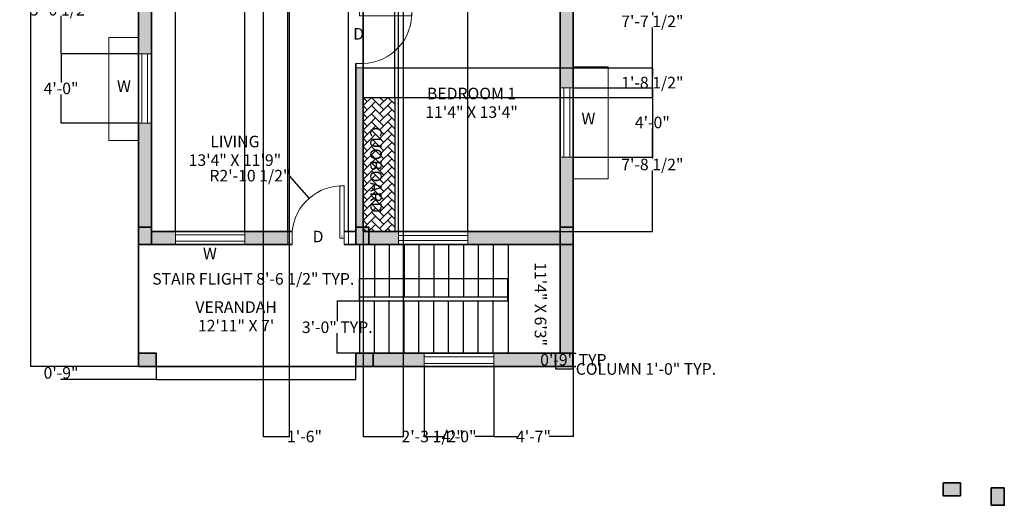
# Model space of a CAD drawing. Units: inches. Extents: x 374 to 1054, y -870 to -188.
# Tile 1 of 3: x 374 to 1054, y -870 to -535. Entities that reach past the tile are written whole.
import ezdxf
from ezdxf.enums import TextEntityAlignment as Align

# ---------------------------------------------------------------- set-up
doc = ezdxf.new("R2010")
doc.units = ezdxf.units.IN
doc.header["$MEASUREMENT"] = 0
for name, color, linetype, lineweight, true_color in [('A-ANNO-DIMS', 244, 'Continuous', 18, 0x991b1e), ('A-AREA-IDEN', 116, 'Continuous', 18, 0x136734), ('A-WALL-PATT', 116, 'Continuous', 13, 0x136734)]:
    doc.layers.add(name, color=color, linetype=linetype, lineweight=lineweight, true_color=true_color)
for name, color, linetype, lineweight in [('A-ANNO-SYMB', 6, 'Continuous', 18), ('A-ANNO-TEXT', 7, 'Continuous', 18), ('A-COLS', 1, 'Continuous', 35), ('A-DOOR', 4, 'Continuous', 18), ('A-FLOR-CASE', 8, 'Continuous', 25), ('A-FLOR-CASE-PATT', 8, 'Continuous', 13), ('A-FLOR-STRS', 7, 'Continuous', 25), ('A-GLAZ', 4, 'Continuous', 18), ('A-GLAZ-PROJ', 4, 'Continuous', 13), ('A-WALL', 7, 'Continuous', 35)]:
    doc.layers.add(name, color=color, linetype=linetype, lineweight=lineweight)
doc.styles.get("Standard").update_dxf_attribs({"font": 'arial.ttf'})
doc.dimstyles.get("Standard").update_dxf_attribs({"dimtxt": 8, "dimasz": 0.18, "dimexe": 0.18, "dimexo": 0.0625, "dimgap": 0.09, "dimtad": 0, "dimtih": 1, "dimtoh": 1, "dimzin": 0, "dimdsep": 46, "dimlunit": 3, "dimtxsty": 'Standard', "dimcen": 0.09, "dimadec": 0, "dimazin": 0, "dimtfac": 1, "dimtofl": 0, "dimtmove": 0, "dimatfit": 3, "dimfxl": 1, "dimtolj": 1, "dimtzin": 0, "dimarcsym": 0})

# ---------------------------------------------------------------- blocks, each defined once
blk = doc.blocks.new('*D2')
at = {"layer": 'A-ANNO-DIMS', "color": 0, "lineweight": -2, "transparency": 16777216}
for p, q in [((455.84, -257.94), (381.2, -257.94)), ((381.38, -258.12), (381.38, -511.76)), ((381.38, -773.76), (381.38, -520.12)), ((455.84, -773.94), (381.2, -773.94))]:
    blk.add_line(p, q, dxfattribs=at)
at = {"layer": 'A-ANNO-DIMS', "color": 0, "transparency": 16777216}
for points in [[(381.35, -258.12), (381.41, -258.12), (381.38, -257.94)], [(381.35, -773.76), (381.41, -773.76), (381.38, -773.94)]]:
    blk.add_solid(points, dxfattribs=at)
at = {"layer": 'Defpoints', "color": 0, "transparency": 16777216}
for p in [(381.38, -257.94), (455.9, -257.94), (455.9, -773.94)]:
    blk.add_point(p, dxfattribs=at)
at = {"layer": 'A-ANNO-DIMS', "color": 0, "transparency": 16777216, "insert": (381.38, -515.94), "char_height": 8, "attachment_point": 5}
blk.add_mtext("\\A1;43'", dxfattribs=at)
blk = doc.blocks.new('COL-12X9')
h = blk.add_hatch(color=256)
h.dxf.hatch_style = 1
h.paths.add_polyline_path([(6, 4.5), (-6, 4.5), (-6, -4.5), (6, -4.5)])
blk.add_lwpolyline([(-6, 4.5), (6, 4.5), (6, -4.5), (-6, -4.5)], close=True)
blk = doc.blocks.new('DOOR-SWING-36')
blk.add_lwpolyline([(0, 0), (-3, 0), (-3, 36), (0, 36)], close=True)
blk.add_arc((-1.5, 1.52), 34.51, 87.5091, 178.37068)
blk = doc.blocks.new('STAIR-FLIGHT-36')
for p, q in [((10.25, 36), (10.25, 0)), ((20.5, 36), (20.5, 0)), ((30.75, 36), (30.75, 0)), ((41, 36), (41, 0)), ((51.25, 36), (51.25, 0)), ((61.5, 36), (61.5, 0)), ((71.75, 36), (71.75, 0)), ((82, 36), (82, 0)), ((92.25, 36), (92.25, 0)), ((0, 0), (102.5, 0))]:
    blk.add_line(p, q)
blk = doc.blocks.new('*D6')
at = {"layer": 'A-ANNO-DIMS', "color": 0, "lineweight": -2, "transparency": 16777216}
for p, q in [((743.74, -774), (743.74, -775.92)), ((755.74, -774), (755.74, -775.92)), ((743.92, -775.74), (755.56, -775.74)), ((755.74, -775.74), (755.92, -775.74))]:
    blk.add_line(p, q, dxfattribs=at)
at = {"layer": 'A-ANNO-DIMS', "color": 0, "transparency": 16777216}
for points in [[(743.92, -775.71), (743.92, -775.77), (743.74, -775.74)], [(755.56, -775.71), (755.56, -775.77), (755.74, -775.74)]]:
    blk.add_solid(points, dxfattribs=at)
at = {"layer": 'Defpoints', "color": 0, "transparency": 16777216}
for p in [(743.74, -773.94), (755.74, -773.94), (755.74, -775.74)]:
    blk.add_point(p, dxfattribs=at)
at = {"layer": 'A-ANNO-DIMS', "color": 0, "transparency": 16777216, "insert": (806.11, -775.74), "char_height": 8, "attachment_point": 5}
blk.add_mtext('\\A1;COLUMN 1\'-0" TYP.', dxfattribs=at)
blk = doc.blocks.new('*D7')
at = {"layer": 'A-ANNO-DIMS', "color": 0, "lineweight": -2, "transparency": 16777216}
for p, q in [((755.8, -764.94), (757.72, -764.94)), ((757.54, -765.12), (757.54, -765.26)), ((755.8, -773.94), (757.72, -773.94)), ((757.54, -773.76), (757.54, -773.61))]:
    blk.add_line(p, q, dxfattribs=at)
at = {"layer": 'A-ANNO-DIMS', "color": 0, "transparency": 16777216}
for points in [[(757.51, -765.12), (757.57, -765.12), (757.54, -764.94)], [(757.51, -773.76), (757.57, -773.76), (757.54, -773.94)]]:
    blk.add_solid(points, dxfattribs=at)
at = {"layer": 'Defpoints', "color": 0, "transparency": 16777216}
for p in [(755.74, -764.94), (757.54, -764.94), (755.74, -773.94)]:
    blk.add_point(p, dxfattribs=at)
at = {"layer": 'A-ANNO-DIMS', "color": 0, "transparency": 16777216, "insert": (757.54, -769.44), "char_height": 8, "attachment_point": 5}
blk.add_mtext('\\A1;0\'-9" TYP.', dxfattribs=at)
blk = doc.blocks.new('*D10')
at = {"layer": 'A-ANNO-DIMS', "color": 0, "lineweight": -2, "transparency": 16777216}
for p, q in [((608.4, -713.56), (608.22, -713.56)), ((608.4, -728.88), (608.4, -713.38)), ((710.72, -713.56), (608.58, -713.56)), ((710.9, -728.88), (710.9, -713.38))]:
    blk.add_line(p, q, dxfattribs=at)
at = {"layer": 'A-ANNO-DIMS', "color": 0, "transparency": 16777216}
for points in [[(608.58, -713.53), (608.58, -713.59), (608.4, -713.56)], [(710.72, -713.53), (710.72, -713.59), (710.9, -713.56)]]:
    blk.add_solid(points, dxfattribs=at)
at = {"layer": 'Defpoints', "color": 0, "transparency": 16777216}
for p in [(608.4, -713.56), (608.4, -728.94), (710.9, -728.94)]:
    blk.add_point(p, dxfattribs=at)
at = {"layer": 'A-ANNO-DIMS', "color": 0, "transparency": 16777216, "insert": (535.02, -713.56), "char_height": 8, "attachment_point": 5}
blk.add_mtext('\\A1;STAIR FLIGHT 8\'-6 1/2" TYP.', dxfattribs=at)
blk = doc.blocks.new('*D11')
at = {"layer": 'A-ANNO-DIMS', "color": 0, "lineweight": -2, "transparency": 16777216}
for p, q in [((608.34, -728.94), (592.85, -728.94)), ((593.03, -729.12), (593.03, -742.76)), ((593.03, -764.76), (593.03, -751.12)), ((608.34, -764.94), (592.85, -764.94))]:
    blk.add_line(p, q, dxfattribs=at)
at = {"layer": 'A-ANNO-DIMS', "color": 0, "transparency": 16777216}
for points in [[(593, -729.12), (593.06, -729.12), (593.03, -728.94)], [(593, -764.76), (593.06, -764.76), (593.03, -764.94)]]:
    blk.add_solid(points, dxfattribs=at)
at = {"layer": 'Defpoints', "color": 0, "transparency": 16777216}
for p in [(608.4, -728.94), (593.03, -764.94), (608.4, -764.94)]:
    blk.add_point(p, dxfattribs=at)
at = {"layer": 'A-ANNO-DIMS', "color": 0, "transparency": 16777216, "insert": (593.03, -746.94), "char_height": 8, "attachment_point": 5}
blk.add_mtext('\\A1;3\'-0" TYP.', dxfattribs=at)
blk = doc.blocks.new('*D22')
at = {"layer": 'A-ANNO-DIMS', "color": 0, "lineweight": -2, "transparency": 16777216}
for p, q in [((455.84, -497.43), (402.18, -497.43)), ((402.36, -497.61), (402.36, -523.56)), ((402.36, -557.96), (402.36, -532.01)), ((455.84, -558.14), (402.18, -558.14))]:
    blk.add_line(p, q, dxfattribs=at)
at = {"layer": 'A-ANNO-DIMS', "color": 0, "transparency": 16777216}
for points in [[(402.33, -497.61), (402.39, -497.61), (402.36, -497.43)], [(402.33, -557.96), (402.39, -557.96), (402.36, -558.14)]]:
    blk.add_solid(points, dxfattribs=at)
at = {"layer": 'Defpoints', "color": 0, "transparency": 16777216}
for p in [(455.9, -497.43), (402.36, -558.14), (455.9, -558.14)]:
    blk.add_point(p, dxfattribs=at)
at = {"layer": 'A-ANNO-DIMS', "color": 0, "transparency": 16777216, "insert": (402.36, -527.79), "char_height": 8, "attachment_point": 5}
blk.add_mtext('\\A1;5\'-0 1/2"', dxfattribs=at)
blk = doc.blocks.new('*D23')
at = {"layer": 'A-ANNO-DIMS', "color": 0, "lineweight": -2, "transparency": 16777216}
for p, q in [((455.84, -558.14), (402.18, -558.14)), ((402.36, -558.32), (402.36, -577.97)), ((402.36, -605.96), (402.36, -586.31)), ((455.84, -606.14), (402.18, -606.14))]:
    blk.add_line(p, q, dxfattribs=at)
at = {"layer": 'A-ANNO-DIMS', "color": 0, "transparency": 16777216}
for points in [[(402.33, -558.32), (402.39, -558.32), (402.36, -558.14)], [(402.33, -605.96), (402.39, -605.96), (402.36, -606.14)]]:
    blk.add_solid(points, dxfattribs=at)
at = {"layer": 'Defpoints', "color": 0, "transparency": 16777216}
for p in [(455.9, -558.14), (402.36, -606.14), (455.9, -606.14)]:
    blk.add_point(p, dxfattribs=at)
at = {"layer": 'A-ANNO-DIMS', "color": 0, "transparency": 16777216, "insert": (402.36, -582.14), "char_height": 8, "attachment_point": 5}
blk.add_mtext('\\A1;4\'-0"', dxfattribs=at)
blk = doc.blocks.new('*D30')
at = {"layer": 'A-ANNO-DIMS', "color": 0, "lineweight": -2, "transparency": 16777216}
for p, q in [((755.97, -489.99), (810.73, -489.99)), ((810.55, -490.17), (810.55, -531.58)), ((810.55, -581.43), (810.55, -540.03)), ((755.97, -581.61), (810.73, -581.61))]:
    blk.add_line(p, q, dxfattribs=at)
at = {"layer": 'A-ANNO-DIMS', "color": 0, "transparency": 16777216}
for points in [[(810.52, -490.17), (810.58, -490.17), (810.55, -489.99)], [(810.52, -581.43), (810.58, -581.43), (810.55, -581.61)]]:
    blk.add_solid(points, dxfattribs=at)
at = {"layer": 'Defpoints', "color": 0, "transparency": 16777216}
for p in [(755.9, -489.99), (755.9, -581.61), (810.55, -581.61)]:
    blk.add_point(p, dxfattribs=at)
at = {"layer": 'A-ANNO-DIMS', "color": 0, "transparency": 16777216, "insert": (810.55, -535.8), "char_height": 8, "attachment_point": 5}
blk.add_mtext('\\A1;7\'-7 1/2"', dxfattribs=at)
blk = doc.blocks.new('*D31')
at = {"layer": 'A-ANNO-DIMS', "color": 0, "lineweight": -2, "transparency": 16777216}
for p, q in [((755.97, -581.61), (810.73, -581.61)), ((810.55, -581.79), (810.55, -601.44)), ((810.55, -629.43), (810.55, -609.79)), ((755.97, -629.61), (810.73, -629.61))]:
    blk.add_line(p, q, dxfattribs=at)
at = {"layer": 'A-ANNO-DIMS', "color": 0, "transparency": 16777216}
for points in [[(810.52, -581.79), (810.58, -581.79), (810.55, -581.61)], [(810.52, -629.43), (810.58, -629.43), (810.55, -629.61)]]:
    blk.add_solid(points, dxfattribs=at)
at = {"layer": 'Defpoints', "color": 0, "transparency": 16777216}
for p in [(755.9, -581.61), (755.9, -629.61), (810.55, -629.61)]:
    blk.add_point(p, dxfattribs=at)
at = {"layer": 'A-ANNO-DIMS', "color": 0, "transparency": 16777216, "insert": (810.55, -605.61), "char_height": 8, "attachment_point": 5}
blk.add_mtext('\\A1;4\'-0"', dxfattribs=at)
blk = doc.blocks.new('*D32')
at = {"layer": 'A-ANNO-DIMS', "color": 0, "lineweight": -2, "transparency": 16777216}
for p, q in [((701.11, -774), (701.11, -822.55)), ((755.9, -774), (755.9, -822.55)), ((701.29, -822.37), (717.62, -822.37)), ((755.72, -822.37), (739.39, -822.37))]:
    blk.add_line(p, q, dxfattribs=at)
at = {"layer": 'A-ANNO-DIMS', "color": 0, "transparency": 16777216}
for points in [[(701.29, -822.34), (701.29, -822.4), (701.11, -822.37)], [(755.72, -822.34), (755.72, -822.4), (755.9, -822.37)]]:
    blk.add_solid(points, dxfattribs=at)
at = {"layer": 'Defpoints', "color": 0, "transparency": 16777216}
for p in [(701.11, -773.94), (755.9, -773.94), (701.11, -822.37)]:
    blk.add_point(p, dxfattribs=at)
at = {"layer": 'A-ANNO-DIMS', "color": 0, "transparency": 16777216, "insert": (728.5, -822.37), "char_height": 8, "attachment_point": 5}
blk.add_mtext('\\A1;4\'-7"', dxfattribs=at)
blk = doc.blocks.new('*D33')
at = {"layer": 'A-ANNO-DIMS', "color": 0, "lineweight": -2, "transparency": 16777216}
for p, q in [((653.11, -774), (653.11, -822.55)), ((701.11, -774), (701.11, -822.55)), ((653.29, -822.37), (666.22, -822.37)), ((700.93, -822.37), (687.99, -822.37))]:
    blk.add_line(p, q, dxfattribs=at)
at = {"layer": 'A-ANNO-DIMS', "color": 0, "transparency": 16777216}
for points in [[(653.29, -822.34), (653.29, -822.4), (653.11, -822.37)], [(700.93, -822.34), (700.93, -822.4), (701.11, -822.37)]]:
    blk.add_solid(points, dxfattribs=at)
at = {"layer": 'Defpoints', "color": 0, "transparency": 16777216}
for p in [(653.11, -773.94), (701.11, -773.94), (653.11, -822.37)]:
    blk.add_point(p, dxfattribs=at)
at = {"layer": 'A-ANNO-DIMS', "color": 0, "transparency": 16777216, "insert": (677.11, -822.37), "char_height": 8, "attachment_point": 5}
blk.add_mtext('\\A1;4\'-0"', dxfattribs=at)
blk = doc.blocks.new('*D34')
at = {"layer": 'A-ANNO-DIMS', "color": 0, "lineweight": -2, "transparency": 16777216}
for p, q in [((467.84, -773.94), (402.18, -773.94)), ((402.36, -774.12), (402.36, -774.26)), ((467.84, -782.94), (402.18, -782.94)), ((402.36, -782.76), (402.36, -782.61))]:
    blk.add_line(p, q, dxfattribs=at)
at = {"layer": 'A-ANNO-DIMS', "color": 0, "transparency": 16777216}
for points in [[(402.33, -774.12), (402.39, -774.12), (402.36, -773.94)], [(402.33, -782.76), (402.39, -782.76), (402.36, -782.94)]]:
    blk.add_solid(points, dxfattribs=at)
at = {"layer": 'Defpoints', "color": 0, "transparency": 16777216}
for p in [(402.36, -773.94), (467.9, -773.94), (467.9, -782.94)]:
    blk.add_point(p, dxfattribs=at)
at = {"layer": 'A-ANNO-DIMS', "color": 0, "transparency": 16777216, "insert": (402.36, -778.44), "char_height": 8, "attachment_point": 5}
blk.add_mtext('\\A1;0\'-9"', dxfattribs=at)
blk = doc.blocks.new('*D35')
at = {"layer": 'A-ANNO-DIMS', "color": 0, "lineweight": -2, "transparency": 16777216}
for p, q in [((610.9, -361.5), (610.9, -822.55)), ((638.56, -361.5), (638.56, -822.55)), ((611.08, -822.37), (638.38, -822.37)), ((638.56, -822.37), (638.74, -822.37))]:
    blk.add_line(p, q, dxfattribs=at)
at = {"layer": 'A-ANNO-DIMS', "color": 0, "transparency": 16777216}
for points in [[(611.08, -822.34), (611.08, -822.4), (610.9, -822.37)], [(638.38, -822.34), (638.38, -822.4), (638.56, -822.37)]]:
    blk.add_solid(points, dxfattribs=at)
at = {"layer": 'Defpoints', "color": 0, "transparency": 16777216}
for p in [(610.9, -361.44), (638.56, -361.44), (638.56, -822.37)]:
    blk.add_point(p, dxfattribs=at)
at = {"layer": 'A-ANNO-DIMS', "color": 0, "transparency": 16777216, "insert": (658.85, -822.37), "char_height": 8, "attachment_point": 5}
blk.add_mtext('\\A1;2\'-3 1/2"', dxfattribs=at)
blk = doc.blocks.new('*D37')
at = {"layer": 'A-ANNO-DIMS', "color": 0, "lineweight": -2, "transparency": 16777216}
for p, q in [((610.9, -588.25), (610.9, -207.66)), ((611.08, -207.84), (632.5, -207.84)), ((632.68, -588.25), (632.68, -207.66)), ((632.68, -207.84), (632.86, -207.84))]:
    blk.add_line(p, q, dxfattribs=at)
at = {"layer": 'A-ANNO-DIMS', "color": 0, "transparency": 16777216}
for points in [[(611.08, -207.81), (611.08, -207.87), (610.9, -207.84)], [(632.5, -207.81), (632.5, -207.87), (632.68, -207.84)]]:
    blk.add_solid(points, dxfattribs=at)
at = {"layer": 'Defpoints', "color": 0, "transparency": 16777216}
for p in [(632.68, -207.84), (610.9, -588.31), (632.68, -588.31)]:
    blk.add_point(p, dxfattribs=at)
at = {"layer": 'A-ANNO-DIMS', "color": 0, "transparency": 16777216, "insert": (646.31, -207.84), "char_height": 8, "attachment_point": 5}
blk.add_mtext('\\A1;1\'-10"', dxfattribs=at)
blk = doc.blocks.new('*D38')
at = {"layer": 'A-ANNO-DIMS', "color": 0, "lineweight": -2, "transparency": 16777216}
for p, q in [((632.74, -588.31), (810.73, -588.31)), ((810.55, -588.49), (810.55, -630.4)), ((810.55, -680.76), (810.55, -638.85)), ((632.74, -680.94), (810.73, -680.94))]:
    blk.add_line(p, q, dxfattribs=at)
at = {"layer": 'A-ANNO-DIMS', "color": 0, "transparency": 16777216}
for points in [[(810.52, -588.49), (810.58, -588.49), (810.55, -588.31)], [(810.52, -680.76), (810.58, -680.76), (810.55, -680.94)]]:
    blk.add_solid(points, dxfattribs=at)
at = {"layer": 'Defpoints', "color": 0, "transparency": 16777216}
for p in [(632.68, -588.31), (632.68, -680.94), (810.55, -680.94)]:
    blk.add_point(p, dxfattribs=at)
at = {"layer": 'A-ANNO-DIMS', "color": 0, "transparency": 16777216, "insert": (810.55, -634.63), "char_height": 8, "attachment_point": 5}
blk.add_mtext('\\A1;7\'-8 1/2"', dxfattribs=at)
blk = doc.blocks.new('*D39')
at = {"layer": 'A-ANNO-DIMS', "color": 0, "lineweight": -2, "transparency": 16777216}
for p, q in [((464.9, -680.88), (464.9, -207.66)), ((465.08, -207.84), (481.13, -207.84)), ((481.31, -680.88), (481.31, -207.66)), ((481.31, -207.84), (481.49, -207.84))]:
    blk.add_line(p, q, dxfattribs=at)
at = {"layer": 'A-ANNO-DIMS', "color": 0, "transparency": 16777216}
for points in [[(465.08, -207.81), (465.08, -207.87), (464.9, -207.84)], [(481.13, -207.81), (481.13, -207.87), (481.31, -207.84)]]:
    blk.add_solid(points, dxfattribs=at)
at = {"layer": 'Defpoints', "color": 0, "transparency": 16777216}
for p in [(481.31, -207.84), (464.9, -680.94), (481.31, -680.94)]:
    blk.add_point(p, dxfattribs=at)
at = {"layer": 'A-ANNO-DIMS', "color": 0, "transparency": 16777216, "insert": (501.16, -207.84), "char_height": 8, "attachment_point": 5}
blk.add_mtext('\\A1;1\'-4 1/2"', dxfattribs=at)
blk = doc.blocks.new('*D40')
at = {"layer": 'A-ANNO-DIMS', "color": 0, "lineweight": -2, "transparency": 16777216}
for p, q in [((481.31, -680.88), (481.31, -207.66)), ((481.49, -207.84), (494.43, -207.84)), ((529.13, -207.84), (516.2, -207.84)), ((529.31, -680.88), (529.31, -207.66))]:
    blk.add_line(p, q, dxfattribs=at)
at = {"layer": 'A-ANNO-DIMS', "color": 0, "transparency": 16777216}
for points in [[(481.49, -207.81), (481.49, -207.87), (481.31, -207.84)], [(529.13, -207.81), (529.13, -207.87), (529.31, -207.84)]]:
    blk.add_solid(points, dxfattribs=at)
at = {"layer": 'Defpoints', "color": 0, "transparency": 16777216}
for p in [(529.31, -207.84), (481.31, -680.94), (529.31, -680.94)]:
    blk.add_point(p, dxfattribs=at)
at = {"layer": 'A-ANNO-DIMS', "color": 0, "transparency": 16777216, "insert": (505.31, -207.84), "char_height": 8, "attachment_point": 5}
blk.add_mtext('\\A1;4\'-0"', dxfattribs=at)
blk = doc.blocks.new('*D41')
at = {"layer": 'A-ANNO-DIMS', "color": 0, "lineweight": -2, "transparency": 16777216}
for p, q in [((529.31, -680.88), (529.31, -207.66)), ((529.49, -207.84), (558.72, -207.84)), ((558.9, -680.88), (558.9, -207.66)), ((558.9, -207.84), (559.08, -207.84))]:
    blk.add_line(p, q, dxfattribs=at)
at = {"layer": 'A-ANNO-DIMS', "color": 0, "transparency": 16777216}
for points in [[(529.49, -207.81), (529.49, -207.87), (529.31, -207.84)], [(558.72, -207.81), (558.72, -207.87), (558.9, -207.84)]]:
    blk.add_solid(points, dxfattribs=at)
at = {"layer": 'Defpoints', "color": 0, "transparency": 16777216}
for p in [(558.9, -207.84), (529.31, -680.94), (558.9, -680.94)]:
    blk.add_point(p, dxfattribs=at)
at = {"layer": 'A-ANNO-DIMS', "color": 0, "transparency": 16777216, "insert": (579.2, -207.84), "char_height": 8, "attachment_point": 5}
blk.add_mtext('\\A1;2\'-5 1/2"', dxfattribs=at)
blk = doc.blocks.new('*D42')
at = {"layer": 'A-ANNO-DIMS', "color": 0, "lineweight": -2, "transparency": 16777216}
for p, q in [((558.9, -680.88), (558.9, -207.66)), ((559.08, -207.84), (569.18, -207.84)), ((600.72, -207.84), (590.63, -207.84)), ((600.9, -680.88), (600.9, -207.66))]:
    blk.add_line(p, q, dxfattribs=at)
at = {"layer": 'A-ANNO-DIMS', "color": 0, "transparency": 16777216}
for points in [[(559.08, -207.81), (559.08, -207.87), (558.9, -207.84)], [(600.72, -207.81), (600.72, -207.87), (600.9, -207.84)]]:
    blk.add_solid(points, dxfattribs=at)
at = {"layer": 'Defpoints', "color": 0, "transparency": 16777216}
for p in [(600.9, -207.84), (558.9, -680.94), (600.9, -680.94)]:
    blk.add_point(p, dxfattribs=at)
at = {"layer": 'A-ANNO-DIMS', "color": 0, "transparency": 16777216, "insert": (579.9, -207.84), "char_height": 8, "attachment_point": 5}
blk.add_mtext('\\A1;3\'-6"', dxfattribs=at)
blk = doc.blocks.new('*D43')
at = {"layer": 'A-ANNO-DIMS', "color": 0, "lineweight": -2, "transparency": 16777216}
for p, q in [((635.25, -680.88), (635.25, -207.66)), ((635.43, -207.84), (648.36, -207.84)), ((683.07, -207.84), (670.13, -207.84)), ((683.25, -680.88), (683.25, -207.66))]:
    blk.add_line(p, q, dxfattribs=at)
at = {"layer": 'A-ANNO-DIMS', "color": 0, "transparency": 16777216}
for points in [[(635.43, -207.81), (635.43, -207.87), (635.25, -207.84)], [(683.07, -207.81), (683.07, -207.87), (683.25, -207.84)]]:
    blk.add_solid(points, dxfattribs=at)
at = {"layer": 'Defpoints', "color": 0, "transparency": 16777216}
for p in [(683.25, -207.84), (635.25, -680.94), (683.25, -680.94)]:
    blk.add_point(p, dxfattribs=at)
at = {"layer": 'A-ANNO-DIMS', "color": 0, "transparency": 16777216, "insert": (659.25, -207.84), "char_height": 8, "attachment_point": 5}
blk.add_mtext('\\A1;4\'-0"', dxfattribs=at)
blk = doc.blocks.new('*D44')
at = {"layer": 'A-ANNO-DIMS', "color": 0, "lineweight": -2, "transparency": 16777216}
for p, q in [((683.25, -680.88), (683.25, -207.66)), ((683.43, -207.84), (695.03, -207.84)), ((746.72, -207.84), (735.12, -207.84)), ((746.9, -680.88), (746.9, -207.66))]:
    blk.add_line(p, q, dxfattribs=at)
at = {"layer": 'A-ANNO-DIMS', "color": 0, "transparency": 16777216}
for points in [[(683.43, -207.81), (683.43, -207.87), (683.25, -207.84)], [(746.72, -207.81), (746.72, -207.87), (746.9, -207.84)]]:
    blk.add_solid(points, dxfattribs=at)
at = {"layer": 'Defpoints', "color": 0, "transparency": 16777216}
for p in [(746.9, -207.84), (683.25, -680.94), (746.9, -680.94)]:
    blk.add_point(p, dxfattribs=at)
at = {"layer": 'A-ANNO-DIMS', "color": 0, "transparency": 16777216, "insert": (715.08, -207.84), "char_height": 8, "attachment_point": 5}
blk.add_mtext('\\A1;5\'-3 1/2"', dxfattribs=at)
blk = doc.blocks.new('*D45')
at = {"layer": 'A-ANNO-DIMS', "color": 0, "lineweight": -2, "transparency": 16777216}
for p, q in [((541.9, -344), (541.9, -822.55)), ((559.9, -344), (559.9, -822.55)), ((542.08, -822.37), (559.72, -822.37)), ((559.9, -822.37), (560.08, -822.37))]:
    blk.add_line(p, q, dxfattribs=at)
at = {"layer": 'A-ANNO-DIMS', "color": 0, "transparency": 16777216}
for points in [[(542.08, -822.34), (542.08, -822.4), (541.9, -822.37)], [(559.72, -822.34), (559.72, -822.4), (559.9, -822.37)]]:
    blk.add_solid(points, dxfattribs=at)
at = {"layer": 'Defpoints', "color": 0, "transparency": 16777216}
for p in [(541.9, -343.94), (559.9, -343.94), (559.9, -822.37)]:
    blk.add_point(p, dxfattribs=at)
at = {"layer": 'A-ANNO-DIMS', "color": 0, "transparency": 16777216, "insert": (570.43, -822.37), "char_height": 8, "attachment_point": 5}
blk.add_mtext('\\A1;1\'-6"', dxfattribs=at)
blk = doc.blocks.new('*D49')
at = {"layer": 'A-ANNO-DIMS', "color": 0, "lineweight": -2, "transparency": 16777216}
for p, q in [((610.97, -567.94), (810.73, -567.94)), ((810.55, -568.12), (810.55, -573.9)), ((810.55, -588.13), (810.55, -582.35)), ((610.97, -588.31), (810.73, -588.31))]:
    blk.add_line(p, q, dxfattribs=at)
at = {"layer": 'A-ANNO-DIMS', "color": 0, "transparency": 16777216}
for points in [[(810.52, -568.12), (810.58, -568.12), (810.55, -567.94)], [(810.52, -588.13), (810.58, -588.13), (810.55, -588.31)]]:
    blk.add_solid(points, dxfattribs=at)
at = {"layer": 'Defpoints', "color": 0, "transparency": 16777216}
for p in [(610.9, -567.94), (610.9, -588.31), (810.55, -588.31)]:
    blk.add_point(p, dxfattribs=at)
at = {"layer": 'A-ANNO-DIMS', "color": 0, "transparency": 16777216, "insert": (810.55, -578.13), "char_height": 8, "attachment_point": 5}
blk.add_mtext('\\A1;1\'-8 1/2"', dxfattribs=at)
blk = doc.blocks.new('*D50')
at = {"layer": 'A-ANNO-DIMS', "color": 0, "lineweight": -2, "transparency": 16777216}
for p, q in [((559.73, -642.34), (559.91, -642.34)), ((559.91, -642.34), (573.48, -657.84)), ((596.31, -684.05), (596.49, -684.05)), ((596.4, -684.14), (596.4, -683.96))]:
    blk.add_line(p, q, dxfattribs=at)
at = {"layer": 'A-ANNO-DIMS', "color": 0, "transparency": 16777216}
blk.add_solid([(573.5, -657.82), (573.45, -657.86), (573.59, -657.98)], dxfattribs=at)
at = {"layer": 'Defpoints', "color": 0, "transparency": 16777216}
for p in [(573.59, -657.98), (596.4, -684.05)]:
    blk.add_point(p, dxfattribs=at)
at = {"layer": 'A-ANNO-DIMS', "color": 0, "transparency": 16777216, "insert": (532.75, -642.34), "char_height": 8, "attachment_point": 5}
blk.add_mtext('\\A1;R2\'-10 1/2"', dxfattribs=at)

msp = doc.modelspace()

# ---------------------------------------------------------------- hatches: boundary and pattern name
at = {"layer": 'A-FLOR-CASE-PATT'}
h = msp.add_hatch(dxfattribs=at)
h.set_pattern_fill('AR-HBONE', color=256)
h.paths.add_polyline_path([(638.563, -266.938), (610.905, -266.938), (610.905, -343.938), (610.905, -361.438), (638.563, -361.438)])
h.paths.add_polyline_path([(620.136, -288.822), (620.136, -356.301), (632.553, -356.301), (632.553, -288.822)], flags=24)
h.paths.add_polyline_path([(727.152, -700.465), (727.152, -761.497), (739.414, -761.497), (739.414, -700.465)], flags=9)
h.paths.add_polyline_path([(497.837, -702.053), (512.386, -702.053), (512.386, -690.053), (497.837, -690.053)], flags=9)
h.paths.add_polyline_path([(494.709, -751.886), (551.702, -751.886), (551.702, -739.837), (494.709, -739.837)], flags=9)
h.paths.add_polyline_path([(490.155, -739.027), (556.256, -739.027), (556.256, -727.027), (490.155, -727.027)], flags=9)
h.paths.add_polyline_path([(488.741, -637.8), (555.988, -637.8), (555.988, -625.538), (488.741, -625.538)], flags=9)
h.paths.add_polyline_path([(501.975, -624.968), (542.755, -624.968), (542.755, -612.559), (501.975, -612.559)], flags=9)
h.paths.add_polyline_path([(498.568, -470.79), (565.812, -470.79), (565.812, -458.536), (498.568, -458.536)], flags=9)
h.paths.add_polyline_path([(510.563, -457.965), (553.816, -457.965), (553.816, -445.555), (510.563, -445.555)], flags=9)
h.paths.add_polyline_path([(474.841, -376.354), (525.689, -376.354), (525.689, -364.092), (474.841, -364.092)], flags=9)
h.paths.add_polyline_path([(483.939, -363.488), (516.591, -363.488), (516.591, -351.283), (483.939, -351.283)], flags=9)
h.paths.add_polyline_path([(652.121, -604.662), (719.368, -604.662), (719.368, -592.4), (652.121, -592.4)], flags=9)
h.paths.add_polyline_path([(650.141, -591.831), (721.347, -591.831), (721.347, -579.414), (650.141, -579.414)], flags=9)
h.paths.add_polyline_path([(613.577, -603.955), (613.577, -672.673), (625.995, -672.673), (625.995, -603.955)], flags=9)
h.paths.add_polyline_path([(704.619, -508.492), (742.954, -508.492), (742.954, -496.492), (704.619, -496.492)], flags=9)
h.paths.add_polyline_path([(706.883, -495.641), (740.69, -495.641), (740.69, -483.641), (706.883, -483.641)], flags=9)
h.paths.add_polyline_path([(695.312, -483.057), (752.261, -483.057), (752.261, -470.566), (695.312, -470.566)], flags=9)
h.paths.add_polyline_path([(699.358, -470.143), (748.215, -470.143), (748.215, -457.734), (699.358, -457.734)], flags=9)
h.paths.add_polyline_path([(623.681, -465.885), (684.71, -465.885), (684.71, -453.631), (623.681, -453.631)], flags=9)
h.paths.add_polyline_path([(611.019, -455.848), (697.775, -455.848), (697.775, -443.357), (611.019, -443.357)], flags=9)
h.paths.add_polyline_path([(625.622, -442.934), (683.172, -442.934), (683.172, -430.525), (625.622, -430.525)], flags=9)
h = msp.add_hatch(dxfattribs=at)
h.set_pattern_fill('AR-HBONE', color=256)
h.paths.add_polyline_path([(632.678, -588.314), (610.905, -588.314), (610.905, -680.938), (632.678, -680.938)])
h.paths.add_polyline_path([(613.577, -603.955), (613.577, -672.673), (625.995, -672.673), (625.995, -603.955)], flags=24)
at = {"layer": 'A-WALL-PATT'}
h = msp.add_hatch(color=256, dxfattribs=at)
h.dxf.hatch_style = 1
h.paths.add_polyline_path([(667.71, -257.938), (614.905, -257.938), (614.905, -266.938), (667.71, -266.938)])
h.paths.add_polyline_path([(746.905, -257.938), (715.71, -257.938), (715.71, -266.938), (746.905, -266.938)])
h.paths.add_polyline_path([(755.905, -270.034), (746.905, -270.034), (746.905, -327.137), (755.905, -327.137)])
h.paths.add_polyline_path([(755.905, -375.137), (746.905, -375.137), (746.905, -422.975), (755.905, -422.975)])
h.paths.add_polyline_path([(605.905, -257.938), (567.481, -257.938), (567.481, -266.938), (605.905, -266.938)])
h.paths.add_polyline_path([(519.481, -257.938), (464.905, -257.938), (464.905, -266.938), (519.481, -266.938)])
h.paths.add_polyline_path([(464.905, -270.108), (455.905, -270.108), (455.905, -285.73), (464.905, -285.73)])
h.paths.add_polyline_path([(464.905, -343.938), (559.905, -343.938), (559.905, -338.938), (464.905, -338.938), (464.905, -333.73), (455.905, -333.73), (455.905, -353.908), (464.905, -353.908)])
h.paths.add_polyline_path([(464.905, -394.938), (541.859, -394.938), (541.863, -389.942), (536.905, -389.938), (464.905, -389.938), (455.905, -389.908), (455.905, -423.118), (464.905, -423.118)])
h.paths.add_polyline_path([(464.905, -435.118), (455.905, -435.118), (455.905, -449.434), (464.905, -449.434)])
h.paths.add_polyline_path([(464.905, -497.434), (455.905, -497.434), (455.905, -515.926), (464.905, -515.926)])
h.paths.add_polyline_path([(464.905, -527.926), (455.905, -527.926), (455.905, -558.14), (464.905, -558.14)])
h.paths.add_polyline_path([(755.905, -489.995), (746.905, -489.995), (746.905, -515.947), (755.905, -515.947)])
h.paths.add_polyline_path([(755.905, -434.975), (746.905, -434.975), (746.905, -453.995), (755.905, -453.995)])
h.paths.add_polyline_path([(746.905, -422.938), (738.905, -422.938), (738.905, -427.938), (746.905, -427.938)])
h.paths.add_polyline_path([(614.905, -423.118), (614.905, -435.118), (605.905, -435.118), (605.905, -423.118), (605.905, -417.938), (610.905, -417.938), (610.905, -423.118)])
h.paths.add_polyline_path([(610.905, -435.118), (605.905, -435.118), (605.905, -469.938), (610.905, -469.938)])
h.paths.add_polyline_path([(541.859, -515.938), (464.905, -515.938), (464.905, -520.938), (541.859, -520.938)])
h.paths.add_polyline_path([(755.905, -527.947), (746.905, -527.947), (746.905, -581.613), (755.905, -581.613)])
h.paths.add_polyline_path([(755.905, -629.613), (746.905, -629.613), (746.905, -677.938), (755.905, -677.938)])
h.paths.add_polyline_path([(755.905, -689.938), (746.905, -689.938), (746.905, -764.938), (755.905, -764.938)])
h.paths.add_polyline_path([(746.905, -680.938), (683.247, -680.938), (683.247, -689.938), (746.905, -689.938)])
h.paths.add_polyline_path([(743.737, -764.938), (701.105, -764.938), (701.105, -773.938), (743.737, -773.938)])
h.paths.add_polyline_path([(653.105, -764.938), (617.905, -764.938), (617.905, -773.938), (653.105, -773.938)])
h.paths.add_polyline_path([(635.247, -680.938), (614.944, -680.938), (614.944, -689.938), (635.247, -689.938)])
h.paths.add_polyline_path([(610.905, -567.938), (605.905, -567.938), (605.905, -677.938), (610.905, -677.938)])
h.paths.add_polyline_path([(558.905, -680.938), (529.314, -680.938), (529.314, -687.485), (529.314, -689.938), (558.905, -689.938)])
h.paths.add_polyline_path([(481.314, -680.938), (464.905, -680.938), (464.905, -689.938), (481.314, -689.938)])
h.paths.add_polyline_path([(464.905, -606.14), (455.905, -606.14), (455.905, -677.938), (464.905, -677.938)])
h.paths.add_polyline_path([(601.753, -550.416), (613.824, -550.416), (613.824, -538.416), (601.753, -538.416)], flags=9)
h.paths.add_polyline_path([(604.254, -492.526), (616.325, -492.526), (616.325, -480.526), (604.254, -480.526)], flags=9)
h.paths.add_polyline_path([(604.661, -400.451), (616.732, -400.451), (616.732, -388.451), (604.661, -388.451)], flags=9)
h.paths.add_polyline_path([(533.025, -378.901), (545.096, -378.901), (545.096, -366.901), (533.025, -366.901)], flags=9)
h.paths.add_polyline_path([(575.128, -346.003), (587.199, -346.003), (587.199, -334.003), (575.128, -334.003)], flags=9)
h.paths.add_polyline_path([(488.741, -637.8), (555.988, -637.8), (555.988, -625.538), (488.741, -625.538)], flags=9)
h.paths.add_polyline_path([(501.975, -624.968), (542.755, -624.968), (542.755, -612.559), (501.975, -612.559)], flags=9)
h.paths.add_polyline_path([(498.568, -470.79), (565.812, -470.79), (565.812, -458.536), (498.568, -458.536)], flags=9)
h.paths.add_polyline_path([(510.563, -457.965), (553.816, -457.965), (553.816, -445.555), (510.563, -445.555)], flags=9)
h.paths.add_polyline_path([(474.841, -376.354), (525.689, -376.354), (525.689, -364.092), (474.841, -364.092)], flags=9)
h.paths.add_polyline_path([(483.939, -363.488), (516.591, -363.488), (516.591, -351.283), (483.939, -351.283)], flags=9)
h.paths.add_polyline_path([(652.121, -604.662), (719.368, -604.662), (719.368, -592.4), (652.121, -592.4)], flags=9)
h.paths.add_polyline_path([(650.141, -591.831), (721.347, -591.831), (721.347, -579.414), (650.141, -579.414)], flags=9)
h.paths.add_polyline_path([(715.698, -427.661), (727.769, -427.661), (727.769, -415.661), (715.698, -415.661)], flags=9)
h.paths.add_polyline_path([(573.757, -690.34), (585.828, -690.34), (585.828, -678.34), (573.757, -678.34)], flags=9)
h.paths.add_polyline_path([(727.152, -700.465), (727.152, -761.497), (739.414, -761.497), (739.414, -700.465)], flags=9)
h.paths.add_polyline_path([(497.837, -702.053), (512.386, -702.053), (512.386, -690.053), (497.837, -690.053)], flags=9)
h.paths.add_polyline_path([(494.709, -751.886), (551.702, -751.886), (551.702, -739.837), (494.709, -739.837)], flags=9)
h.paths.add_polyline_path([(490.155, -739.027), (556.256, -739.027), (556.256, -727.027), (490.155, -727.027)], flags=9)
h.paths.add_polyline_path([(613.577, -603.955), (613.577, -672.673), (625.995, -672.673), (625.995, -603.955)], flags=9)
h.paths.add_polyline_path([(695.312, -483.057), (752.261, -483.057), (752.261, -470.566), (695.312, -470.566)], flags=9)
h.paths.add_polyline_path([(611.019, -455.848), (697.775, -455.848), (697.775, -443.357), (611.019, -443.357)], flags=9)
h.paths.add_polyline_path([(663.069, -377.631), (720.133, -377.631), (720.133, -365.369), (663.069, -365.369)], flags=9)
h.paths.add_polyline_path([(657.829, -364.537), (729.035, -364.537), (729.035, -352.12), (657.829, -352.12)], flags=9)
h.paths.add_polyline_path([(620.136, -288.822), (620.136, -356.301), (632.553, -356.301), (632.553, -288.822)], flags=9)
h.paths.add_polyline_path([(497.968, -305.851), (548.814, -305.851), (548.814, -293.597), (497.968, -293.597)], flags=9)
h.paths.add_polyline_path([(496.797, -293.026), (549.986, -293.026), (549.986, -280.617), (496.797, -280.617)], flags=9)
h = msp.add_hatch(color=256, dxfattribs=at)
h.dxf.hatch_style = 1
h.paths.add_polyline_path([(705.905, -425.438), (705.905, -422.938), (610.905, -422.938), (610.905, -417.938), (605.905, -417.938), (605.905, -469.938), (610.905, -469.938), (610.905, -435.118), (610.905, -427.938), (693.905, -427.938), (698.905, -427.938), (705.905, -427.938)])
h.paths.add_polyline_path([(715.698, -427.661), (727.769, -427.661), (727.769, -415.661), (715.698, -415.661)], flags=9)
h.paths.add_polyline_path([(573.757, -690.34), (585.828, -690.34), (585.828, -678.34), (573.757, -678.34)], flags=9)
h.paths.add_polyline_path([(601.753, -550.416), (613.824, -550.416), (613.824, -538.416), (601.753, -538.416)], flags=9)
h.paths.add_polyline_path([(604.254, -492.526), (616.325, -492.526), (616.325, -480.526), (604.254, -480.526)], flags=9)
h.paths.add_polyline_path([(604.661, -400.451), (616.732, -400.451), (616.732, -388.451), (604.661, -388.451)], flags=9)
h.paths.add_polyline_path([(533.025, -378.901), (545.096, -378.901), (545.096, -366.901), (533.025, -366.901)], flags=9)
h.paths.add_polyline_path([(575.128, -346.003), (587.199, -346.003), (587.199, -334.003), (575.128, -334.003)], flags=9)
h.paths.add_polyline_path([(727.152, -700.465), (727.152, -761.497), (739.414, -761.497), (739.414, -700.465)], flags=9)
h.paths.add_polyline_path([(497.837, -702.053), (512.386, -702.053), (512.386, -690.053), (497.837, -690.053)], flags=9)
h.paths.add_polyline_path([(494.709, -751.886), (551.702, -751.886), (551.702, -739.837), (494.709, -739.837)], flags=9)
h.paths.add_polyline_path([(490.155, -739.027), (556.256, -739.027), (556.256, -727.027), (490.155, -727.027)], flags=9)
h.paths.add_polyline_path([(488.741, -637.8), (555.988, -637.8), (555.988, -625.538), (488.741, -625.538)], flags=9)
h.paths.add_polyline_path([(501.975, -624.968), (542.755, -624.968), (542.755, -612.559), (501.975, -612.559)], flags=9)
h.paths.add_polyline_path([(498.568, -470.79), (565.812, -470.79), (565.812, -458.536), (498.568, -458.536)], flags=9)
h.paths.add_polyline_path([(510.563, -457.965), (553.816, -457.965), (553.816, -445.555), (510.563, -445.555)], flags=9)
h.paths.add_polyline_path([(474.841, -376.354), (525.689, -376.354), (525.689, -364.092), (474.841, -364.092)], flags=9)
h.paths.add_polyline_path([(483.939, -363.488), (516.591, -363.488), (516.591, -351.283), (483.939, -351.283)], flags=9)
h.paths.add_polyline_path([(652.121, -604.662), (719.368, -604.662), (719.368, -592.4), (652.121, -592.4)], flags=9)
h.paths.add_polyline_path([(650.141, -591.831), (721.347, -591.831), (721.347, -579.414), (650.141, -579.414)], flags=9)
h.paths.add_polyline_path([(613.577, -603.955), (613.577, -672.673), (625.995, -672.673), (625.995, -603.955)], flags=9)
h.paths.add_polyline_path([(704.619, -508.492), (742.954, -508.492), (742.954, -496.492), (704.619, -496.492)], flags=9)
h.paths.add_polyline_path([(706.883, -495.641), (740.69, -495.641), (740.69, -483.641), (706.883, -483.641)], flags=9)
h.paths.add_polyline_path([(695.312, -483.057), (752.261, -483.057), (752.261, -470.566), (695.312, -470.566)], flags=9)
h.paths.add_polyline_path([(699.358, -470.143), (748.215, -470.143), (748.215, -457.734), (699.358, -457.734)], flags=9)
h.paths.add_polyline_path([(623.681, -465.885), (684.71, -465.885), (684.71, -453.631), (623.681, -453.631)], flags=25)
h.paths.add_polyline_path([(611.019, -455.848), (697.775, -455.848), (697.775, -443.357), (611.019, -443.357)], flags=25)
h.paths.add_polyline_path([(625.622, -442.934), (683.172, -442.934), (683.172, -430.525), (625.622, -430.525)], flags=25)
h.paths.add_polyline_path([(663.069, -377.631), (720.133, -377.631), (720.133, -365.369), (663.069, -365.369)], flags=9)
h.paths.add_polyline_path([(657.829, -364.537), (729.035, -364.537), (729.035, -352.12), (657.829, -352.12)], flags=9)
h.paths.add_polyline_path([(620.136, -288.822), (620.136, -356.301), (632.553, -356.301), (632.553, -288.822)], flags=9)
h.paths.add_polyline_path([(497.968, -305.851), (548.814, -305.851), (548.814, -293.597), (497.968, -293.597)], flags=9)
h.paths.add_polyline_path([(496.797, -293.026), (549.986, -293.026), (549.986, -280.617), (496.797, -280.617)], flags=9)

# ---------------------------------------------------------------- linework, layer by layer
at = {"layer": 'A-ANNO-SYMB'}
for points in [[(601.147, -707.938, 0, 0, 0), (671.71, -707.938, 6, 0, 0), (680.155, -707.938, 0, 0, 0), (720.71, -707.938, 0, 0, 0), (720.71, -746.687, 0, 0, 0), (649.405, -746.687, 6, 0, 0), (642.259, -746.687, 0, 0, 0)], [(536.018, -791.976, 0, 0, 0), (536.018, -768.241, 6, 0, 0), (536.018, -760.492, 0, 0, 0)]]:
    msp.add_lwpolyline(points, format="xyseb", dxfattribs=at)
at = {"layer": 'A-DOOR'}
for p, q in [((610.905, -564.938), (605.905, -564.938)), ((610.905, -567.938), (605.905, -567.938)), ((558.905, -680.938), (558.905, -689.938)), ((561.905, -680.938), (561.905, -689.938)), ((597.905, -680.938), (597.905, -689.938)), ((600.905, -680.938), (600.905, -689.938))]:
    msp.add_line(p, q, dxfattribs=at)
msp.add_lwpolyline([(597.905, -685.438), (594.905, -685.438), (594.905, -649.438), (597.905, -649.438)], close=True, dxfattribs=at)
msp.add_arc((596.405, -684.045), 34.64, 87.518145, 174.853705, dxfattribs=at)
at = {"layer": 'A-FLOR-CASE'}
for p, q in [((610.905, -588.314), (632.678, -588.314)), ((632.678, -588.314), (632.678, -680.938))]:
    msp.add_line(p, q, dxfattribs=at)
at = {"layer": 'A-FLOR-STRS'}
for p, q in [((608.405, -689.938), (608.405, -764.938)), ((710.905, -689.938), (710.905, -764.938)), ((467.905, -773.938), (467.905, -782.938)), ((605.905, -782.938), (605.905, -773.938)), ((467.905, -782.938), (605.905, -782.938))]:
    msp.add_line(p, q, dxfattribs=at)
at = {"layer": 'A-GLAZ'}
for p, q in [((464.905, -558.14), (455.905, -558.14)), ((458.054, -606.14), (458.054, -558.14)), ((462.122, -606.14), (462.122, -558.14)), ((746.905, -581.613), (755.905, -581.613)), ((749.46, -629.613), (749.46, -581.613)), ((753.492, -581.613), (753.492, -629.613)), ((464.905, -606.14), (455.905, -606.14)), ((746.905, -629.613), (755.905, -629.613)), ((481.314, -680.938), (481.314, -689.938)), ((529.314, -683.269), (481.314, -683.269)), ((529.314, -680.938), (529.314, -689.938)), ((635.247, -680.938), (635.247, -689.938)), ((635.247, -683.625), (683.247, -683.625)), ((683.247, -680.938), (683.247, -689.938)), ((481.314, -687.485), (529.314, -687.485)), ((683.247, -687.187), (635.247, -687.187)), ((653.105, -764.938), (653.105, -773.938)), ((653.105, -767.44), (701.105, -767.44)), ((701.105, -764.938), (701.105, -773.938)), ((701.105, -772.036), (653.105, -772.036))]:
    msp.add_line(p, q, dxfattribs=at)
at = {"layer": 'A-GLAZ-PROJ'}
for p, q in [((455.905, -547.018), (435.35, -547.018)), ((435.35, -547.018), (435.35, -618.024)), ((755.905, -567.296), (780.16, -567.296)), ((780.16, -567.296), (780.16, -644.422)), ((435.35, -618.024), (455.905, -618.024)), ((780.16, -644.422), (755.905, -644.422))]:
    msp.add_line(p, q, dxfattribs=at)
at = {"layer": 'A-WALL'}
for p, q in [((464.905, -680.938), (464.905, -394.938)), ((746.905, -520.938), (746.905, -680.938)), ((605.905, -680.938), (605.905, -564.938)), ((610.905, -680.938), (610.905, -564.938)), ((464.905, -680.938), (561.905, -680.938)), ((597.905, -680.938), (605.905, -680.938)), ((610.905, -680.938), (746.905, -680.938)), ((455.905, -689.938), (561.905, -689.938)), ((597.905, -689.938), (746.905, -689.938)), ((746.905, -689.938), (746.905, -764.938)), ((746.905, -764.938), (605.905, -764.938)), ((605.905, -764.938), (605.905, -773.938))]:
    msp.add_line(p, q, dxfattribs=at)
msp.add_lwpolyline([(455.905, -257.938), (755.905, -257.938), (755.905, -773.938), (455.905, -773.938)], close=True, dxfattribs=at)

# ---------------------------------------------------------------- block references
at = {"layer": 'A-COLS'}
for p, rotation in [((460.405, -683.938), 269.9999999999991), ((610.444, -683.938), 269.9999999999994), ((751.405, -683.938), 269.9999999999983), ((1049.023, -863.844), 269.9999999999988)]:
    msp.add_blockref('COL-12X9', p, dxfattribs=dict(at, rotation=rotation))
for p in [(461.905, -769.438), (611.905, -769.438), (749.737, -769.438), (1017.235, -858.754)]:
    msp.add_blockref('COL-12X9', p, dxfattribs=at)
at = {"layer": 'A-DOOR', "extrusion": (0, 0, -1), "zscale": -1, "rotation": 89.99999999999989}
msp.add_blockref('DOOR-SWING-36', (-608.405, -528.938), dxfattribs=at)
at = {"layer": 'A-FLOR-STRS'}
msp.add_blockref('STAIR-FLIGHT-36', (608.405, -725.938), dxfattribs=at)
at = {"layer": 'A-FLOR-STRS', "rotation": 180}
msp.add_blockref('STAIR-FLIGHT-36', (710.905, -728.938), dxfattribs=at)

# ---------------------------------------------------------------- texts
at = {"layer": 'A-ANNO-TEXT'}
for s, p in [('D', (607.789, -548.416)), ('W', (445.787, -584.544)), ('W', (766.402, -606.951)), ('D', (579.792, -688.34)), ('W', (505.111, -700.053))]:
    msp.add_text(s, height=8, dxfattribs=at).set_placement(p, align=Align.CENTER)
msp.add_text('CUOBOARD', height=8, rotation=270, dxfattribs=at).set_placement((615.783, -638.314), align=Align.CENTER)
at = {"layer": 'A-AREA-IDEN'}
for s, p in [('BEDROOM 1', (685.744, -589.625)), ('11\'4" X 13\'4"', (685.744, -602.477)), ('LIVING', (522.365, -622.764)), ('13\'4" X 11\'9"', (522.365, -635.615)), ('VERANDAH', (523.206, -737.027)), ('12\'11" X 7\'', (523.206, -749.878))]:
    msp.add_text(s, height=8, dxfattribs=at).set_placement(p, align=Align.CENTER)
msp.add_text('11\'4" X 6\'3"', height=8, rotation=270, dxfattribs=at).set_placement((729.338, -730.981), align=Align.CENTER)

# ---------------------------------------------------------------- dimensions: what is measured, and where the dimension line sits
at = {"layer": 'A-ANNO-DIMS'}
for base, p1, p2, picture, middle in [((481.314, -207.841), (464.905, -680.938), (481.314, -680.938), '*D39', (501.161, -207.841)), ((558.905, -207.841), (529.314, -680.938), (558.905, -680.938), '*D41', (579.197, -207.841)), ((746.905, -207.841), (683.247, -680.938), (746.905, -680.938), '*D44', (715.076, -207.841)), ((529.314, -207.841), (481.314, -680.938), (529.314, -680.938), '*D40', (505.314, -207.841)), ((600.905, -207.841), (558.905, -680.938), (600.905, -680.938), '*D42', (579.905, -207.841)), ((632.678, -207.841), (610.905, -588.314), (632.678, -588.314), '*D37', (646.312, -207.841)), ((683.247, -207.841), (635.247, -680.938), (683.247, -680.938), '*D43', (659.247, -207.841)), ((559.905, -822.366), (541.905, -343.938), (559.905, -343.938), '*D45', (570.431, -822.366)), ((638.563, -822.366), (610.905, -361.438), (638.563, -361.438), '*D35', (658.855, -822.366)), ((653.105, -822.366), (701.105, -773.938), (653.105, -773.938), '*D33', (677.105, -822.366)), ((701.105, -822.366), (755.905, -773.938), (701.105, -773.938), '*D32', (728.505, -822.366))]:
    dim = msp.add_linear_dim(base=base, p1=p1, p2=p2, dimstyle='Standard', override={"dimdec": 1, "dimlfac": 1, "dimrnd": 0, "dimzin": 1, "dimdsep": 46, "dimlunit": 4, "dimfrac": 2}, dxfattribs=at)
    dim.commit()
    dim.dimension.update_dxf_attribs({"geometry": picture, "text_midpoint": middle})
for base, p1, p2, override, picture, middle in [((381.378, -257.938), (455.905, -773.938), (455.905, -257.938), {"dimclrd": 0, "dimclre": 0, "dimclrt": 0}, '*D2', (381.378, -515.938)), ((810.55, -581.613), (755.905, -489.995), (755.905, -581.613), {"dimdec": 1, "dimlfac": 1, "dimrnd": 0, "dimzin": 1, "dimdsep": 46, "dimlunit": 4, "dimfrac": 2}, '*D30', (810.55, -535.804)), ((402.361, -558.14), (455.905, -497.434), (455.905, -558.14), {"dimdec": 1, "dimlfac": 1, "dimrnd": 0, "dimzin": 1, "dimdsep": 46, "dimlunit": 4, "dimfrac": 2}, '*D22', (402.361, -527.787)), ((402.361, -606.14), (455.905, -558.14), (455.905, -606.14), {"dimdec": 1, "dimlfac": 1, "dimrnd": 0, "dimzin": 1, "dimdsep": 46, "dimlunit": 4, "dimfrac": 2}, '*D23', (402.361, -582.14)), ((810.55, -588.314), (610.905, -567.938), (610.905, -588.314), {"dimdec": 1, "dimlfac": 1, "dimrnd": 0, "dimzin": 1, "dimdsep": 46, "dimlunit": 4, "dimfrac": 2}, '*D49', (810.55, -578.126)), ((810.55, -629.613), (755.905, -581.613), (755.905, -629.613), {"dimdec": 1, "dimlfac": 1, "dimrnd": 0, "dimzin": 1, "dimdsep": 46, "dimlunit": 4, "dimfrac": 2}, '*D31', (810.55, -605.613)), ((810.55, -680.938), (632.678, -588.314), (632.678, -680.938), {"dimdec": 1, "dimlfac": 1, "dimrnd": 0, "dimzin": 1, "dimdsep": 46, "dimlunit": 4, "dimfrac": 2}, '*D38', (810.55, -634.626)), ((402.361, -773.938), (467.905, -782.938), (467.905, -773.938), {"dimdec": 1, "dimlfac": 1, "dimrnd": 0, "dimzin": 1, "dimdsep": 46, "dimlunit": 4, "dimfrac": 2}, '*D34', (402.361, -778.438))]:
    dim = msp.add_linear_dim(base=base, p1=p1, p2=p2, angle=90, dimstyle='Standard', override=override, dxfattribs=at)
    dim.commit()
    dim.dimension.update_dxf_attribs({"geometry": picture, "text_midpoint": middle})
dim = msp.add_radius_dim(center=(596.405, -684.045), mpoint=(573.594, -657.976), dimstyle='Standard', override={"dimdec": 1, "dimlfac": 1, "dimrnd": 0, "dimzin": 1, "dimdsep": 46, "dimlunit": 4, "dimfrac": 2}, dxfattribs=at)
dim.commit()
dim.dimension.update_dxf_attribs({"geometry": '*D50', "text_midpoint": (532.748, -642.335), "dimtype": 164})
for base, p1, p2, angle, text, picture, middle in [((608.405, -713.563), (710.905, -728.938), (608.405, -728.938), 180, 'STAIR FLIGHT <> TYP.', '*D10', (535.022, -713.563)), ((593.03, -764.938), (608.405, -728.938), (608.405, -764.938), 270, '<> TYP.', '*D11', (593.03, -746.938)), ((757.537, -764.938), (755.737, -773.938), (755.737, -764.938), 90, '<> TYP.', '*D7', (757.537, -769.438))]:
    dim = msp.add_linear_dim(base=base, p1=p1, p2=p2, angle=angle, text=text, dimstyle='Standard', override={"dimdec": 1, "dimlfac": 1, "dimrnd": 0, "dimzin": 1, "dimdsep": 46, "dimlunit": 4, "dimfrac": 2}, dxfattribs=at)
    dim.commit()
    dim.dimension.update_dxf_attribs({"geometry": picture, "text_midpoint": middle})
dim = msp.add_linear_dim(base=(755.737, -775.738), p1=(743.737, -773.938), p2=(755.737, -773.938), text='COLUMN <> TYP.', dimstyle='Standard', override={"dimdec": 1, "dimlfac": 1, "dimrnd": 0, "dimzin": 1, "dimdsep": 46, "dimlunit": 4, "dimfrac": 2}, dxfattribs=at)
dim.commit()
dim.dimension.update_dxf_attribs({"geometry": '*D6', "text_midpoint": (806.11, -775.738)})

doc.saveas('drawing.dxf')
